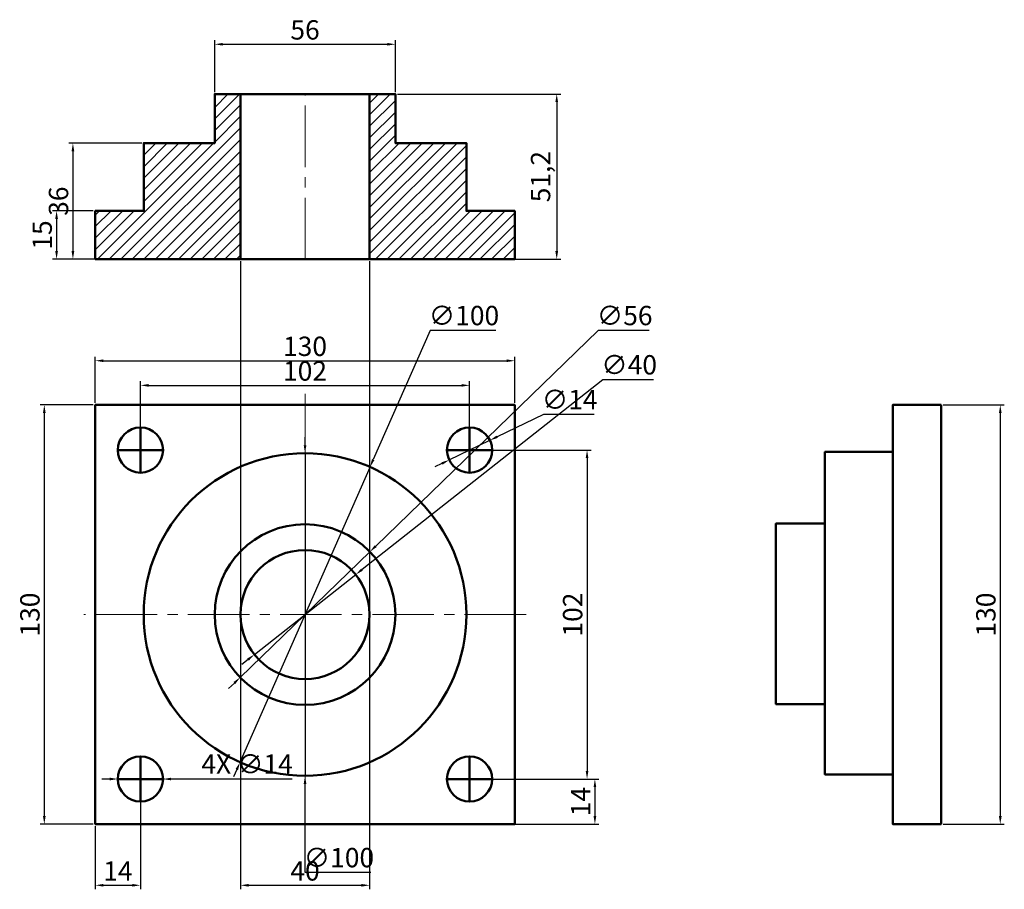
# Model space of a CAD drawing. Units: millimetres. Extents: x 22 to 327, y -2 to 267.
import ezdxf

# ---------------------------------------------------------------- set-up
doc = ezdxf.new("R2010")
doc.units = ezdxf.units.MM
doc.linetypes.add('CENTER2', pattern=[28.575, 19.05, -3.175, 3.175, -3.175])
for name, color, linetype, lineweight in [('M-CNTR', 4, 'CENTER2', 18), ('M-DIMS', 2, 'Continuous', 25), ('M-HATC', 8, 'Continuous', 18), ('M-OUTL', 7, 'Continuous', 50)]:
    doc.layers.add(name, color=color, linetype=linetype, lineweight=lineweight)
doc.styles.get("Standard").update_dxf_attribs({"font": 'arial.ttf'})
doc.dimstyles.new('ISO-25', dxfattribs={"dimtxt": 6, "dimasz": 2.5, "dimexe": 1.25, "dimexo": 0.625, "dimtad": 1, "dimtoh": 1, "dimdec": 1, "dimtxsty": 'Standard', "dimcen": 2.5, "dimadec": 0, "dimazin": 0, "dimtfac": 1, "dimtdec": 1, "dimtmove": 0, "dimatfit": 3, "dimfxl": 1, "dimarcsym": 0})

# ---------------------------------------------------------------- blocks, each defined once
blk = doc.blocks.new('*D1')
at = {"layer": 'Defpoints', "color": 0, "transparency": 16777216}
for p in [(307.22, 147.84), (307.22, 17.84), (325.55, 17.84)]:
    blk.add_point(p, dxfattribs=at)
at = {"layer": 'M-DIMS', "color": 0, "lineweight": -2, "transparency": 16777216}
for p, q in [((307.85, 147.84), (326.8, 147.84)), ((325.55, 145.34), (325.55, 20.34)), ((307.85, 17.84), (326.8, 17.84))]:
    blk.add_line(p, q, dxfattribs=at)
at = {"layer": 'M-DIMS', "color": 0, "transparency": 16777216}
for points in [[(325.13, 145.34), (325.97, 145.34), (325.55, 147.84)], [(325.13, 20.34), (325.97, 20.34), (325.55, 17.84)]]:
    blk.add_solid(points, dxfattribs=at)
at = {"layer": 'M-DIMS', "color": 0, "transparency": 16777216, "insert": (321.86, 82.84), "char_height": 6, "attachment_point": 5, "rotation": 90}
blk.add_mtext('130', dxfattribs=at)
blk = doc.blocks.new('*D2')
at = {"layer": 'Defpoints', "color": 0, "transparency": 16777216}
for p in [(175.08, 161.55), (45.08, 147.84), (175.08, 147.84)]:
    blk.add_point(p, dxfattribs=at)
at = {"layer": 'M-DIMS', "color": 0, "lineweight": -2, "transparency": 16777216}
for p, q in [((45.08, 148.46), (45.08, 162.8)), ((175.08, 148.46), (175.08, 162.8)), ((47.58, 161.55), (172.58, 161.55))]:
    blk.add_line(p, q, dxfattribs=at)
at = {"layer": 'M-DIMS', "color": 0, "transparency": 16777216}
for points in [[(47.58, 161.97), (47.58, 161.14), (45.08, 161.55)], [(172.58, 161.97), (172.58, 161.14), (175.08, 161.55)]]:
    blk.add_solid(points, dxfattribs=at)
at = {"layer": 'M-DIMS', "color": 0, "transparency": 16777216, "insert": (110.08, 165.25), "char_height": 6, "attachment_point": 5}
blk.add_mtext('130', dxfattribs=at)
blk = doc.blocks.new('*D3')
at = {"layer": 'Defpoints', "color": 0, "transparency": 16777216}
for p in [(161.08, 153.92), (59.08, 133.84), (161.08, 133.84)]:
    blk.add_point(p, dxfattribs=at)
at = {"layer": 'M-DIMS', "color": 0, "lineweight": -2, "transparency": 16777216}
for p, q in [((59.08, 134.46), (59.08, 155.17)), ((61.58, 153.92), (158.58, 153.92)), ((161.08, 134.46), (161.08, 155.17))]:
    blk.add_line(p, q, dxfattribs=at)
at = {"layer": 'M-DIMS', "color": 0, "transparency": 16777216}
for points in [[(61.58, 154.33), (61.58, 153.5), (59.08, 153.92)], [(158.58, 154.33), (158.58, 153.5), (161.08, 153.92)]]:
    blk.add_solid(points, dxfattribs=at)
at = {"layer": 'M-DIMS', "color": 0, "transparency": 16777216, "insert": (110.08, 157.6), "char_height": 6, "attachment_point": 5}
blk.add_mtext('102', dxfattribs=at)
blk = doc.blocks.new('*D4')
at = {"layer": 'Defpoints', "color": 0, "transparency": 16777216}
for p in [(45.08, 147.84), (29.28, 17.84), (45.08, 17.84)]:
    blk.add_point(p, dxfattribs=at)
at = {"layer": 'M-DIMS', "color": 0, "lineweight": -2, "transparency": 16777216}
for p, q in [((44.46, 147.84), (28.03, 147.84)), ((29.28, 145.34), (29.28, 20.34)), ((44.46, 17.84), (28.03, 17.84))]:
    blk.add_line(p, q, dxfattribs=at)
at = {"layer": 'M-DIMS', "color": 0, "transparency": 16777216}
for points in [[(28.86, 145.34), (29.7, 145.34), (29.28, 147.84)], [(28.86, 20.34), (29.7, 20.34), (29.28, 17.84)]]:
    blk.add_solid(points, dxfattribs=at)
at = {"layer": 'M-DIMS', "color": 0, "transparency": 16777216, "insert": (25.59, 82.84), "char_height": 6, "attachment_point": 5, "rotation": 90}
blk.add_mtext('130', dxfattribs=at)
blk = doc.blocks.new('*D5')
at = {"layer": 'Defpoints', "color": 0, "transparency": 16777216}
for p in [(161.08, 133.84), (161.08, 31.84), (197.49, 31.84)]:
    blk.add_point(p, dxfattribs=at)
at = {"layer": 'M-DIMS', "color": 0, "lineweight": -2, "transparency": 16777216}
for p, q in [((161.71, 133.84), (198.74, 133.84)), ((197.49, 131.34), (197.49, 34.34)), ((161.71, 31.84), (198.74, 31.84))]:
    blk.add_line(p, q, dxfattribs=at)
at = {"layer": 'M-DIMS', "color": 0, "transparency": 16777216}
for points in [[(197.07, 131.34), (197.91, 131.34), (197.49, 133.84)], [(197.07, 34.34), (197.91, 34.34), (197.49, 31.84)]]:
    blk.add_solid(points, dxfattribs=at)
at = {"layer": 'M-DIMS', "color": 0, "transparency": 16777216, "insert": (193.8, 82.84), "char_height": 6, "attachment_point": 5, "rotation": 90}
blk.add_mtext('102', dxfattribs=at)
blk = doc.blocks.new('*D6')
at = {"layer": 'Defpoints', "color": 0, "transparency": 16777216}
for p in [(167.39, 136.88), (154.78, 130.79)]:
    blk.add_point(p, dxfattribs=at)
at = {"layer": 'M-DIMS', "color": 0, "lineweight": -2, "transparency": 16777216}
for p, q in [((183.94, 144.89), (169.64, 137.97)), ((199.66, 144.89), (183.94, 144.89)), ((154.78, 130.79), (167.39, 136.88)), ((152.53, 129.7), (150.28, 128.61))]:
    blk.add_line(p, q, dxfattribs=at)
at = {"layer": 'M-DIMS', "color": 0, "transparency": 16777216}
for points in [[(169.45, 138.35), (169.82, 137.6), (167.39, 136.88)], [(152.35, 130.07), (152.71, 129.32), (154.78, 130.79)]]:
    blk.add_solid(points, dxfattribs=at)
at = {"layer": 'M-DIMS', "color": 0, "transparency": 16777216, "insert": (192.11, 148.74), "char_height": 6, "attachment_point": 5}
blk.add_mtext('∅14', dxfattribs=at)
blk = doc.blocks.new('*D7')
at = {"layer": 'Defpoints', "color": 0, "transparency": 16777216}
for p in [(161.08, 31.84), (161.08, 17.84), (199.92, 17.84)]:
    blk.add_point(p, dxfattribs=at)
at = {"layer": 'M-DIMS', "color": 0, "lineweight": -2, "transparency": 16777216}
for p, q in [((161.71, 31.84), (201.17, 31.84)), ((199.92, 29.34), (199.92, 20.34)), ((161.71, 17.84), (201.17, 17.84))]:
    blk.add_line(p, q, dxfattribs=at)
at = {"layer": 'M-DIMS', "color": 0, "transparency": 16777216}
for points in [[(199.51, 29.34), (200.34, 29.34), (199.92, 31.84)], [(199.51, 20.34), (200.34, 20.34), (199.92, 17.84)]]:
    blk.add_solid(points, dxfattribs=at)
at = {"layer": 'M-DIMS', "color": 0, "transparency": 16777216, "insert": (196.28, 24.84), "char_height": 6, "attachment_point": 5, "rotation": 90}
blk.add_mtext('14', dxfattribs=at)
blk = doc.blocks.new('*D8')
at = {"layer": 'Defpoints', "color": 0, "transparency": 16777216}
for p in [(125.78, 95.23), (94.38, 70.45)]:
    blk.add_point(p, dxfattribs=at)
at = {"layer": 'M-DIMS', "color": 0, "lineweight": -2, "transparency": 16777216}
for p, q in [((202.35, 155.65), (127.75, 96.77)), ((218.08, 155.65), (202.35, 155.65)), ((94.38, 70.45), (125.78, 95.23)), ((92.42, 68.9), (90.46, 67.35))]:
    blk.add_line(p, q, dxfattribs=at)
at = {"layer": 'M-DIMS', "color": 0, "transparency": 16777216}
for points in [[(127.49, 97.1), (128, 96.45), (125.78, 95.23)], [(92.16, 69.22), (92.68, 68.57), (94.38, 70.45)]]:
    blk.add_solid(points, dxfattribs=at)
at = {"layer": 'M-DIMS', "color": 0, "transparency": 16777216, "insert": (210.53, 159.51), "char_height": 6, "attachment_point": 5}
blk.add_mtext('∅40', dxfattribs=at)
blk = doc.blocks.new('*D9')
at = {"layer": 'Defpoints', "color": 0, "transparency": 16777216}
for p in [(130.19, 102.32), (89.98, 63.35)]:
    blk.add_point(p, dxfattribs=at)
at = {"layer": 'M-DIMS', "color": 0, "lineweight": -2, "transparency": 16777216}
for p, q in [((200.96, 170.93), (131.98, 104.06)), ((216.71, 170.93), (200.96, 170.93)), ((89.98, 63.35), (130.19, 102.32)), ((88.18, 61.61), (86.39, 59.87))]:
    blk.add_line(p, q, dxfattribs=at)
at = {"layer": 'M-DIMS', "color": 0, "transparency": 16777216}
for points in [[(131.69, 104.36), (132.27, 103.76), (130.19, 102.32)], [(87.89, 61.91), (88.47, 61.31), (89.98, 63.35)]]:
    blk.add_solid(points, dxfattribs=at)
at = {"layer": 'M-DIMS', "color": 0, "transparency": 16777216, "insert": (209.15, 174.79), "char_height": 6, "attachment_point": 5}
blk.add_mtext('∅56', dxfattribs=at)
blk = doc.blocks.new('*D10')
at = {"layer": 'Defpoints', "color": 0, "transparency": 16777216}
for p in [(130.22, 128.6), (89.95, 37.07)]:
    blk.add_point(p, dxfattribs=at)
at = {"layer": 'M-DIMS', "color": 0, "lineweight": -2, "transparency": 16777216}
for p, q in [((148.83, 170.93), (131.22, 130.89)), ((169.22, 170.93), (148.83, 170.93)), ((89.95, 37.07), (130.22, 128.6)), ((88.95, 34.78), (87.94, 32.49))]:
    blk.add_line(p, q, dxfattribs=at)
at = {"layer": 'M-DIMS', "color": 0, "transparency": 16777216}
for points in [[(130.84, 131.06), (131.6, 130.72), (130.22, 128.6)], [(88.56, 34.95), (89.33, 34.61), (89.95, 37.07)]]:
    blk.add_solid(points, dxfattribs=at)
at = {"layer": 'M-DIMS', "color": 0, "transparency": 16777216, "insert": (159.34, 174.79), "char_height": 6, "attachment_point": 5}
blk.add_mtext('∅100', dxfattribs=at)
blk = doc.blocks.new('*D11')
at = {"layer": 'Defpoints', "color": 0, "transparency": 16777216}
for p in [(45.08, 208.04), (33.09, 193.04), (45.08, 193.04)]:
    blk.add_point(p, dxfattribs=at)
at = {"layer": 'M-DIMS', "color": 0, "lineweight": -2, "transparency": 16777216}
for p, q in [((44.46, 208.04), (31.84, 208.04)), ((33.09, 205.54), (33.09, 195.54)), ((44.46, 193.04), (31.84, 193.04))]:
    blk.add_line(p, q, dxfattribs=at)
at = {"layer": 'M-DIMS', "color": 0, "transparency": 16777216}
for points in [[(32.67, 205.54), (33.5, 205.54), (33.09, 208.04)], [(32.67, 195.54), (33.5, 195.54), (33.09, 193.04)]]:
    blk.add_solid(points, dxfattribs=at)
at = {"layer": 'M-DIMS', "color": 0, "transparency": 16777216, "insert": (29.4, 200.54), "char_height": 6, "attachment_point": 5, "rotation": 90}
blk.add_mtext('15', dxfattribs=at)
blk = doc.blocks.new('*D12')
at = {"layer": 'Defpoints', "color": 0, "transparency": 16777216}
for p in [(60.08, 229.04), (38.15, 193.04), (60.08, 193.04)]:
    blk.add_point(p, dxfattribs=at)
at = {"layer": 'M-DIMS', "color": 0, "lineweight": -2, "transparency": 16777216}
for p, q in [((59.46, 229.04), (36.9, 229.04)), ((38.15, 226.54), (38.15, 195.54)), ((59.46, 193.04), (36.9, 193.04))]:
    blk.add_line(p, q, dxfattribs=at)
at = {"layer": 'M-DIMS', "color": 0, "transparency": 16777216}
for points in [[(37.73, 226.54), (38.56, 226.54), (38.15, 229.04)], [(37.73, 195.54), (38.56, 195.54), (38.15, 193.04)]]:
    blk.add_solid(points, dxfattribs=at)
at = {"layer": 'M-DIMS', "color": 0, "transparency": 16777216, "insert": (34.46, 211.04), "char_height": 6, "attachment_point": 5, "rotation": 90}
blk.add_mtext('36', dxfattribs=at)
blk = doc.blocks.new('*D13')
at = {"layer": 'Defpoints', "color": 0, "transparency": 16777216}
for p in [(138.08, 244.24), (138.08, 193.04), (188.09, 193.04)]:
    blk.add_point(p, dxfattribs=at)
at = {"layer": 'M-DIMS', "color": 0, "lineweight": -2, "transparency": 16777216}
for p, q in [((138.71, 244.24), (189.34, 244.24)), ((188.09, 241.74), (188.09, 195.54)), ((138.71, 193.04), (189.34, 193.04))]:
    blk.add_line(p, q, dxfattribs=at)
at = {"layer": 'M-DIMS', "color": 0, "transparency": 16777216}
for points in [[(187.67, 241.74), (188.51, 241.74), (188.09, 244.24)], [(187.67, 195.54), (188.51, 195.54), (188.09, 193.04)]]:
    blk.add_solid(points, dxfattribs=at)
at = {"layer": 'M-DIMS', "color": 0, "transparency": 16777216, "insert": (183.86, 218.64), "char_height": 6, "attachment_point": 5, "rotation": 90}
blk.add_mtext('51,2', dxfattribs=at)
blk = doc.blocks.new('MOUNTING-HOLE-D14')
for p, q in [((0, 7), (0, -7)), ((7, 0), (-7, 0))]:
    blk.add_line(p, q)
blk.add_circle((0, 0), 7)
blk = doc.blocks.new('*D15')
at = {"layer": 'Defpoints', "color": 0, "transparency": 16777216}
for p in [(90.08, 193.04), (130.08, 193.04), (130.08, -1.11)]:
    blk.add_point(p, dxfattribs=at)
at = {"layer": 'M-DIMS', "color": 0, "lineweight": -2, "transparency": 16777216}
for p, q in [((90.08, 192.42), (90.08, -2.36)), ((130.08, 192.42), (130.08, -2.36)), ((92.58, -1.11), (127.58, -1.11))]:
    blk.add_line(p, q, dxfattribs=at)
at = {"layer": 'M-DIMS', "color": 0, "transparency": 16777216}
for points in [[(92.58, -0.7), (92.58, -1.53), (90.08, -1.11)], [(127.58, -0.7), (127.58, -1.53), (130.08, -1.11)]]:
    blk.add_solid(points, dxfattribs=at)
at = {"layer": 'M-DIMS', "color": 0, "transparency": 16777216, "insert": (110.08, 2.57), "char_height": 6, "attachment_point": 5}
blk.add_mtext('40', dxfattribs=at)
blk = doc.blocks.new('*D16')
at = {"layer": 'Defpoints', "color": 0, "transparency": 16777216}
for p in [(138.08, 259.69), (82.08, 244.24), (138.08, 244.24)]:
    blk.add_point(p, dxfattribs=at)
at = {"layer": 'M-DIMS', "color": 0, "lineweight": -2, "transparency": 16777216}
for p, q in [((82.08, 244.87), (82.08, 260.94)), ((84.58, 259.69), (135.58, 259.69)), ((138.08, 244.87), (138.08, 260.94))]:
    blk.add_line(p, q, dxfattribs=at)
at = {"layer": 'M-DIMS', "color": 0, "transparency": 16777216}
for points in [[(84.58, 260.11), (84.58, 259.28), (82.08, 259.69)], [(135.58, 260.11), (135.58, 259.28), (138.08, 259.69)]]:
    blk.add_solid(points, dxfattribs=at)
at = {"layer": 'M-DIMS', "color": 0, "transparency": 16777216, "insert": (110.08, 263.38), "char_height": 6, "attachment_point": 5}
blk.add_mtext('56', dxfattribs=at)
blk = doc.blocks.new('*D17')
at = {"layer": 'Defpoints', "color": 0, "transparency": 16777216}
for p in [(59.08, 31.84), (45.08, 17.84), (59.08, -1.11)]:
    blk.add_point(p, dxfattribs=at)
at = {"layer": 'M-DIMS', "color": 0, "lineweight": -2, "transparency": 16777216}
for p, q in [((59.08, 31.21), (59.08, -2.36)), ((45.08, 17.21), (45.08, -2.36)), ((47.58, -1.11), (56.58, -1.11))]:
    blk.add_line(p, q, dxfattribs=at)
at = {"layer": 'M-DIMS', "color": 0, "transparency": 16777216}
for points in [[(47.58, -0.7), (47.58, -1.53), (45.08, -1.11)], [(56.58, -0.7), (56.58, -1.53), (59.08, -1.11)]]:
    blk.add_solid(points, dxfattribs=at)
at = {"layer": 'M-DIMS', "color": 0, "transparency": 16777216, "insert": (52.08, 2.52), "char_height": 6, "attachment_point": 5}
blk.add_mtext('14', dxfattribs=at)
blk = doc.blocks.new('*D18')
at = {"layer": 'Defpoints', "color": 0, "transparency": 16777216}
for p in [(110.08, 132.84), (110.08, 32.84)]:
    blk.add_point(p, dxfattribs=at)
at = {"layer": 'M-DIMS', "color": 0, "lineweight": -2, "transparency": 16777216}
for p, q in [((110.08, 135.34), (110.08, 137.84)), ((110.08, 132.84), (110.08, 32.84)), ((110.08, 2.84), (110.08, 30.34)), ((130.47, 2.84), (110.08, 2.84))]:
    blk.add_line(p, q, dxfattribs=at)
at = {"layer": 'M-DIMS', "color": 0, "transparency": 16777216}
for points in [[(110.5, 135.34), (109.67, 135.34), (110.08, 132.84)], [(110.5, 30.34), (109.67, 30.34), (110.08, 32.84)]]:
    blk.add_solid(points, dxfattribs=at)
at = {"layer": 'M-DIMS', "color": 0, "transparency": 16777216, "insert": (120.59, 6.69), "char_height": 6, "attachment_point": 5}
blk.add_mtext('∅100', dxfattribs=at)
blk = doc.blocks.new('*D19')
at = {"layer": 'Defpoints', "color": 0, "transparency": 16777216}
for p in [(52.08, 31.84), (66.08, 31.83)]:
    blk.add_point(p, dxfattribs=at)
at = {"layer": 'M-DIMS', "color": 0, "lineweight": -2, "transparency": 16777216}
for p, q in [((49.58, 31.84), (47.08, 31.84)), ((52.08, 31.84), (66.08, 31.83)), ((77.55, 31.83), (68.58, 31.83)), ((106.08, 31.83), (77.55, 31.83))]:
    blk.add_line(p, q, dxfattribs=at)
at = {"layer": 'M-DIMS', "color": 0, "transparency": 16777216}
for points in [[(49.58, 32.25), (49.58, 31.42), (52.08, 31.84)], [(68.58, 32.25), (68.58, 31.42), (66.08, 31.83)]]:
    blk.add_solid(points, dxfattribs=at)
at = {"layer": 'M-DIMS', "color": 0, "transparency": 16777216, "insert": (92.13, 35.69), "char_height": 6, "attachment_point": 5}
blk.add_mtext('4X ∅14', dxfattribs=at)

msp = doc.modelspace()

# ---------------------------------------------------------------- hatches: boundary and pattern name
at = {"layer": 'M-HATC'}
h = msp.add_hatch(dxfattribs=at)
h.set_pattern_fill('ANSI31', color=256, scale=0.8)
h.paths.add_polyline_path([(90.08, 244.24), (82.08, 244.24), (82.08, 229.04), (60.08, 229.04), (60.08, 208.04), (45.08, 208.04), (45.08, 193.04), (90.08, 193.04)])
h.paths.add_polyline_path([(160.08, 229.04), (138.08, 229.04), (138.08, 244.24), (130.08, 244.24), (130.08, 193.04), (175.08, 193.04), (175.08, 208.04), (160.08, 208.04)])

# ---------------------------------------------------------------- linework, layer by layer
at = {"layer": 'M-CNTR'}
for p, q in [((110.08, 193.04), (110.08, 244.24)), ((110.08, 151.34), (110.08, 14.34)), ((178.58, 82.84), (41.58, 82.84))]:
    msp.add_line(p, q, dxfattribs=at)
at = {"layer": 'M-OUTL'}
for p, q in [((90.08, 193.04), (90.08, 244.24)), ((130.08, 193.04), (130.08, 244.24))]:
    msp.add_line(p, q, dxfattribs=at)
for points in [[(45.08, 193.04), (45.08, 208.04), (60.08, 208.04), (60.08, 229.04), (82.08, 229.04), (82.08, 244.24), (138.08, 244.24), (138.08, 229.04), (160.08, 229.04), (160.08, 208.04), (175.08, 208.04), (175.08, 193.04)], [(175.08, 17.84), (175.08, 147.84), (45.08, 147.84), (45.08, 17.84)], [(307.22, 147.84), (307.22, 17.84), (292.22, 17.84), (292.22, 147.84)]]:
    msp.add_lwpolyline(points, close=True, dxfattribs=at)
for points in [[(292.22, 133.27), (271.22, 133.27), (271.22, 33.27), (292.22, 33.27)], [(271.22, 111.07), (256.02, 111.07), (256.02, 55.07), (271.22, 55.07)]]:
    msp.add_lwpolyline(points, dxfattribs=at)
for radius in [50, 28, 20]:
    msp.add_circle((110.08, 82.84), radius, dxfattribs=at)

# ---------------------------------------------------------------- block references
msp.add_blockref('MOUNTING-HOLE-D14', (59.08, 133.84), dxfattribs=at)
for p, rotation in [((161.08, 133.84), 270.0000000000002), ((59.08, 31.84), 89.99999999999982), ((161.08, 31.84), 180)]:
    msp.add_blockref('MOUNTING-HOLE-D14', p, dxfattribs=dict(at, rotation=rotation))

# ---------------------------------------------------------------- dimensions: what is measured, and where the dimension line sits
at = {"layer": 'M-DIMS'}
for base, p1, p2, override, picture, middle in [((138.08, 259.69), (82.08, 244.24), (138.08, 244.24), {"dimdec": 0, "dimlfac": 1, "dimrnd": 0, "dimzin": 0, "dimdsep": 46, "dimlunit": 2}, '*D16', (110.08, 263.38)), ((130.08, -1.11), (90.08, 193.04), (130.08, 193.04), {"dimdec": 0, "dimlfac": 1, "dimrnd": 0, "dimzin": 0, "dimdsep": 46, "dimlunit": 2}, '*D15', (110.08, 2.57)), ((175.08, 161.55), (45.08, 147.84), (175.08, 147.84), {"dimclrd": 0, "dimclre": 0, "dimclrt": 0}, '*D2', (110.08, 165.25)), ((161.08, 153.92), (59.08, 133.84), (161.08, 133.84), {"dimclrd": 0, "dimclre": 0, "dimclrt": 0}, '*D3', (110.08, 157.6)), ((59.08, -1.11), (45.08, 17.84), (59.08, 31.84), {"dimdec": 0, "dimlfac": 1, "dimrnd": 0, "dimzin": 0, "dimdsep": 46, "dimlunit": 2}, '*D17', (52.08, 2.52))]:
    dim = msp.add_linear_dim(base=base, p1=p1, p2=p2, dimstyle='ISO-25', override=override, dxfattribs=at)
    dim.commit()
    dim.dimension.update_dxf_attribs({"geometry": picture, "text_midpoint": middle})
for base, p1, p2, picture, middle in [((188.09, 193.04), (138.08, 244.24), (138.08, 193.04), '*D13', (183.86, 218.64)), ((38.15, 193.04), (60.08, 229.04), (60.08, 193.04), '*D12', (34.46, 211.04)), ((33.09, 193.04), (45.08, 208.04), (45.08, 193.04), '*D11', (29.4, 200.54)), ((29.28, 17.84), (45.08, 147.84), (45.08, 17.84), '*D4', (25.59, 82.84)), ((325.55, 17.84), (307.22, 147.84), (307.22, 17.84), '*D1', (321.86, 82.84)), ((197.49, 31.84), (161.08, 133.84), (161.08, 31.84), '*D5', (193.8, 82.84)), ((199.92, 17.84), (161.08, 31.84), (161.08, 17.84), '*D7', (196.28, 24.84))]:
    dim = msp.add_linear_dim(base=base, p1=p1, p2=p2, angle=90, dimstyle='ISO-25', override={"dimclrd": 0, "dimclre": 0, "dimclrt": 0}, dxfattribs=at)
    dim.commit()
    dim.dimension.update_dxf_attribs({"geometry": picture, "text_midpoint": middle})
for p1, p2, override, picture, middle in [((89.98, 63.35), (130.19, 102.32), {"dimclrd": 0, "dimclre": 0, "dimclrt": 0}, '*D9', (209.15, 170.93)), ((89.95, 37.07), (130.22, 128.6), {"dimclrd": 0, "dimclre": 0, "dimclrt": 0}, '*D10', (159.34, 170.93)), ((94.38, 70.45), (125.78, 95.23), {"dimclrd": 0, "dimclre": 0, "dimclrt": 0}, '*D8', (210.53, 155.65)), ((154.78, 130.79), (167.39, 136.88), {"dimclrd": 0, "dimclre": 0, "dimclrt": 0}, '*D6', (192.11, 144.89)), ((110.08, 132.84), (110.08, 32.84), {"dimdec": 0, "dimlfac": 1, "dimrnd": 0, "dimzin": 0, "dimdsep": 46, "dimlunit": 2}, '*D18', (120.59, 2.84))]:
    dim = msp.add_diameter_dim_2p(p1=p1, p2=p2, dimstyle='ISO-25', override=override, dxfattribs=at)
    dim.commit()
    dim.dimension.update_dxf_attribs({"geometry": picture, "text_midpoint": middle, "dimtype": 163})
dim = msp.add_diameter_dim_2p(p1=(52.08, 31.84), p2=(66.08, 31.84), text='4X <>', dimstyle='ISO-25', override={"dimdec": 0, "dimlfac": 1, "dimrnd": 0, "dimzin": 0, "dimdsep": 46, "dimlunit": 2}, dxfattribs=at)
dim.commit()
dim.dimension.update_dxf_attribs({"geometry": '*D19', "text_midpoint": (77.55, 31.83), "dimtype": 163})

doc.saveas('drawing.dxf')
